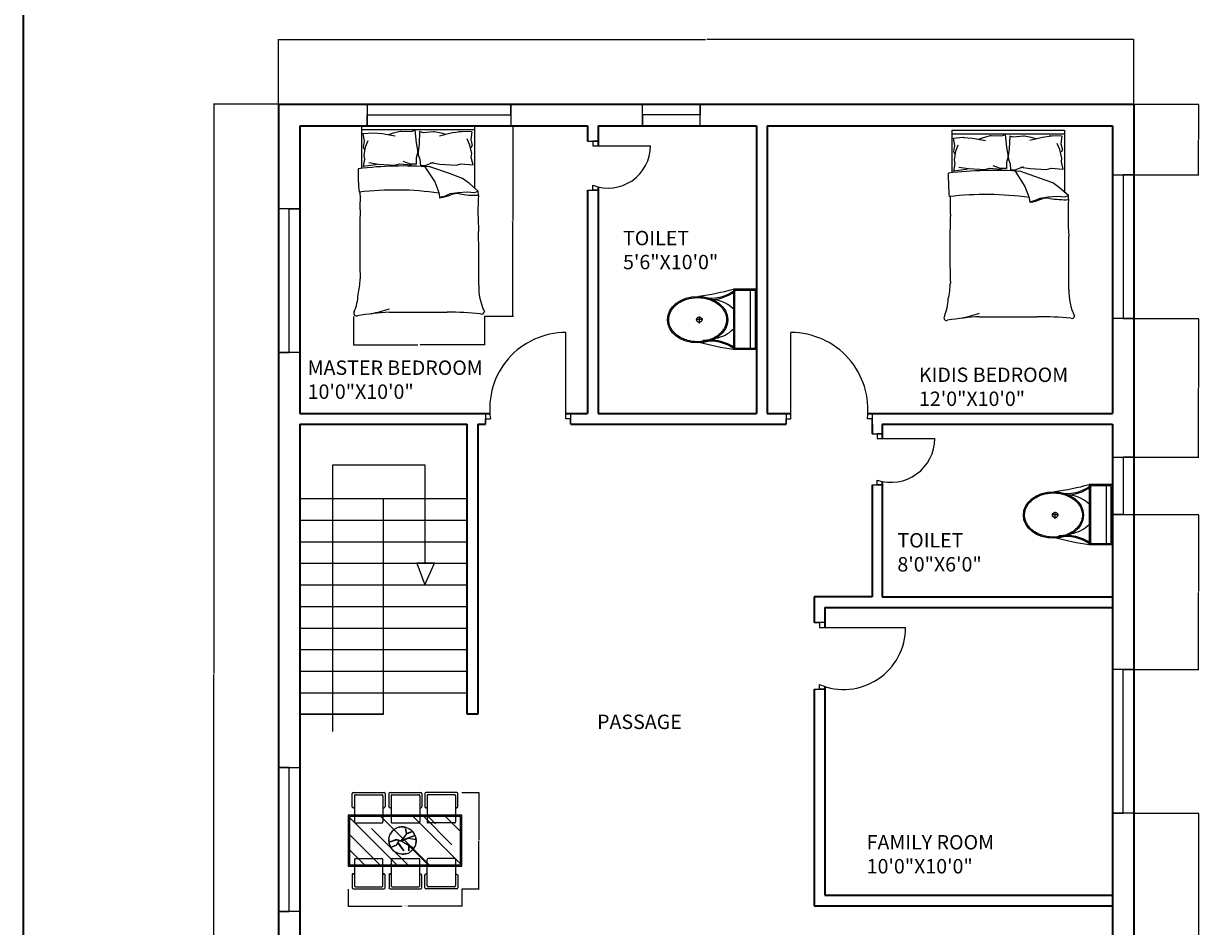
# Model space of a CAD drawing. Units: inches. Extents: x 1912 to 3731, y 1384 to 2459.
# Tile 2 of 8: x 1912 to 2405, y 1630 to 2007. Entities that reach past the tile are written whole.
import ezdxf

# ---------------------------------------------------------------- set-up
doc = ezdxf.new("R2010")
doc.units = ezdxf.units.IN
for name, color, linetype, lineweight in [('A-ANNO-DIMS', 2, 'Continuous', 18), ('A-ANNO-TTLB', 7, 'Continuous', 35), ('A-AREA-IDEN', 7, 'Continuous', 18), ('A-DOOR', 3, 'Continuous', 20), ('A-FLOR-FIXT', 9, 'Continuous', 18), ('A-FLOR-STRS', 7, 'Continuous', 18), ('A-FURN', 8, 'Continuous', 15), ('A-GLAZ', 4, 'Continuous', 18), ('A-WALL', 7, 'Continuous', 35)]:
    doc.layers.add(name, color=color, linetype=linetype, lineweight=lineweight)
doc.styles.get("Standard").update_dxf_attribs({"font": 'arial.ttf'})
doc.dimstyles.get("Standard").update_dxf_attribs({"dimtxt": 0.18, "dimasz": 0.18, "dimexe": 0.18, "dimexo": 0.0625, "dimgap": 0.09, "dimtad": 0, "dimtih": 1, "dimtoh": 1, "dimdec": 4, "dimzin": 0, "dimdsep": 46, "dimtxsty": 'Standard', "dimcen": 0.09, "dimadec": 0, "dimazin": 0, "dimtfac": 1, "dimtdec": 4, "dimtofl": 0, "dimtmove": 0, "dimatfit": 3, "dimfxl": 1, "dimtolj": 1, "dimtzin": 0, "dimarcsym": 0})

# ---------------------------------------------------------------- blocks, each defined once
blk = doc.blocks.new('A$C31115884')
for p, q in [((258, 466), (258, 523)), ((283, 498), (223, 498)), ((0, 200), (0, 0)), ((520, 200), (0, 200)), ((10, 190), (10, 10)), ((510, 190), (10, 190)), ((510, 10), (510, 190)), ((520, 0), (520, 200)), ((510, 54), (0, 54)), ((10, 10), (510, 10)), ((0, 0), (520, 0))]:
    blk.add_line(p, q)
blk.add_circle((256, 496), 23.6)
for centre, radius, start, end in [((2778, -205), 2807, 165.4549, 171.7133), ((-295, 403), 365, 324.2091, 9.3499), ((-295, 403), 375, 324.2091, 9.3499), ((139, 406), 293, 315.8436, 2.6563), ((806, 403), 365, 170.6501, 215.7909), ((3237, 905), 2807, 188.2867, 194.5451), ((384, 406), 293, 190.2774, 224.1564), ((806, 403), 375, 179.2036, 215.7909)]:
    blk.add_arc(centre, radius, start, end)
blk.add_ellipse((256, 510), major_axis=(0, -261), ratio=0.772727)
blk.add_open_spline([(256, 259), (263, 259), (270, 260), (288, 262), (299, 265), (320, 273), (330, 278), (350, 291), (360, 299), (378, 316), (386, 326), (402, 347), (409, 358), (421, 383), (427, 395), (436, 422), (440, 436), (445, 465), (447, 480), (448, 509), (448, 524), (445, 553), (443, 568), (436, 596), (432, 610), (422, 636), (416, 649), (402, 672), (395, 683), (379, 703), (370, 712), (351, 728), (341, 735), (321, 746), (310, 751), (289, 757), (278, 759), (256, 761), (245, 761), (223, 757), (212, 754), (191, 746), (181, 741), (161, 728), (151, 720), (133, 703), (125, 693), (110, 672), (103, 660), (90, 636), (85, 623), (76, 596), (72, 582), (67, 553), (66, 538), (64, 509), (65, 494), (68, 465), (70, 450), (77, 422), (81, 408), (91, 382), (97, 370), (111, 346), (118, 335), (135, 316), (144, 307), (162, 291), (172, 284), (193, 273), (203, 269), (225, 262), (236, 260), (250, 259), (253, 259), (256, 259)], degree=3, knots=[0, 0, 0, 0, 0.110105, 0.110105, 0.285049, 0.285049, 0.459994, 0.459994, 0.634938, 0.634938, 0.809882, 0.809882, 0.984827, 0.984827, 1.159771, 1.159771, 1.334715, 1.334715, 1.50966, 1.50966, 1.684604, 1.684604, 1.859549, 1.859549, 2.034493, 2.034493, 2.209437, 2.209437, 2.384382, 2.384382, 2.559326, 2.559326, 2.73427, 2.73427, 2.909215, 2.909215, 3.084159, 3.084159, 3.259103, 3.259103, 3.434048, 3.434048, 3.608992, 3.608992, 3.783936, 3.783936, 3.958881, 3.958881, 4.133825, 4.133825, 4.30877, 4.30877, 4.483714, 4.483714, 4.658658, 4.658658, 4.833603, 4.833603, 5.008547, 5.008547, 5.183491, 5.183491, 5.358436, 5.358436, 5.53338, 5.53338, 5.708324, 5.708324, 5.883269, 5.883269, 6.058213, 6.058213, 6.233158, 6.233158, 6.283185, 6.283185, 6.283185, 6.283185])
blk = doc.blocks.new('BED-DOUBLE')
for p, q in [((3.41, 61.57), (3.41, 79.35)), ((3.41, 79.35), (50.34, 79.35)), ((50.34, 79.35), (50.34, 53.22)), ((3.41, 77.85), (50.34, 77.85)), ((3.82, 76.1), (4.39, 72.97)), ((3.83, 76.07), (8.03, 76.4)), ((8.03, 76.4), (8.14, 76.38)), ((8.14, 76.38), (11.89, 76.1)), ((11.89, 76.1), (17.29, 75.1)), ((14.59, 75.67), (16.58, 76.38)), ((16.58, 76.38), (19.41, 77.09)), ((19.41, 77.09), (19.73, 77.09)), ((19.73, 77.09), (24.1, 76.95)), ((24.1, 76.95), (25.52, 77.52)), ((25.52, 77.52), (26.08, 72.26)), ((27.47, 76.9), (27.24, 71.63)), ((28.93, 76.43), (27.47, 76.9)), ((33.27, 76.84), (28.93, 76.43)), ((33.59, 76.86), (33.27, 76.84)), ((36.47, 76.33), (33.59, 76.86)), ((41.16, 76.34), (35.84, 75.01)), ((38.5, 75.74), (36.47, 76.33)), ((44.89, 76.86), (41.16, 76.34)), ((49.21, 76.84), (43.91, 76.94)), ((43.91, 76.94), (44.89, 76.86)), ((49.21, 76.84), (48.84, 73.69)), ((4.39, 72.97), (3.97, 70.42)), ((3.97, 70.42), (4.53, 69.42)), ((4.39, 67.01), (4.96, 70.56)), ((4.96, 70.56), (5.95, 73.26)), ((26.08, 72.26), (26.65, 69.14)), ((26.65, 69.14), (26.65, 67.86)), ((27.24, 71.63), (26.86, 68.47)), ((48.42, 71.24), (47.26, 73.87)), ((49.21, 67.74), (48.42, 71.24)), ((48.84, 73.69), (49.42, 71.16)), ((49.42, 71.16), (48.92, 70.14)), ((4.11, 62.32), (4.68, 65.45)), ((4.68, 65.45), (4.39, 67.01)), ((23.67, 63.38), (20.58, 64.45)), ((26.65, 67.86), (26.08, 66.01)), ((26.08, 66.01), (26.08, 63.38)), ((26.86, 68.47), (26.94, 67.2)), ((26.94, 67.2), (27.62, 65.39)), ((27.62, 65.39), (27.79, 62.76)), ((30.2, 62.91), (33.21, 64.17)), ((49.03, 66.16), (49.21, 67.74)), ((49.79, 63.08), (49.03, 66.16)), ((9.11, 63.03), (4.11, 62.32)), ((6.27, 64), (10.23, 63.35)), ((10.23, 63.35), (9.11, 63.03)), ((10.23, 63.35), (17.11, 62.93)), ((17.11, 62.93), (19.04, 63.47)), ((19.04, 63.47), (24.08, 63.08)), ((26.08, 63.38), (23.67, 63.38)), ((27.79, 62.76), (30.2, 62.91)), ((29.72, 62.28), (33.83, 55.9)), ((39.91, 59.4), (31.73, 62.28)), ((31.98, 64), (35.94, 63.35)), ((35.94, 63.35), (42.82, 62.93)), ((45.39, 57.42), (39.91, 59.4)), ((42.82, 62.93), (44.75, 63.47)), ((44.75, 63.47), (49.79, 63.08)), ((33.83, 55.9), (35.5, 51.5)), ((48.28, 55.3), (45.39, 57.42)), ((51.92, 52.1), (48.28, 55.3)), ((35.5, 51.5), (35.81, 49.52)), ((35.81, 49.52), (38.24, 50.13)), ((38.24, 50.13), (40.22, 51.04)), ((40.22, 51.04), (43.56, 51.5)), ((43.56, 51.5), (47.37, 51.8)), ((47.37, 51.8), (50.41, 51.5)), ((50.41, 51.5), (51.92, 52.1)), ((52, 50.39), (51.92, 52.1, 3.8)), ((14.79, 1.53), (38.96, 1.53))]:
    blk.add_line(p, q)
for centre, radius, start, end in [((83.63, 59.62), 81.81, 178.7218, 185.604), ((20.98, -99.43), 162, 86.0865, 96.7821), ((17.44, -74.15), 126.7, 81.7845, 96.9006), ((-164.3, 48.74), 167.05, 358.4762, 1.0082), ((35.98, 49.46), 0.181, 160.2464, 271.1377), ((30.59, 77.9), 29.12, 280.6617, 289.8806), ((42.96, 44.92), 6.11, 78.6608, 113.7384), ((50.4, 85.89), 35.53, 259.8763, 272.5657), ((178.99, 43.69), 127.17, 176.9791, 183.8365), ((476.11, 29.65), 473.64, 178.2277, 181.7185), ((-4427.7, 12.75), 4479.86, 0.00217, 0.28689), ((-26.42, 16), 29.1, 346.0648, 358.9113), ((74.79, 11.92), 22.65, 177.4714, 206.4681), ((-21.27, 10.34), 23.14, 337.9751, 356.652), ((1.07, 1.07), 1.07, 146.1736, 293.4781), ((21.04, -117.88), 119.57, 92.9958, 99.4091), ((-16.91, 102.64), 104.55, 283.3832, 287.7053), ((40.41, -129.11), 130.65, 84.4998, 90.6351), ((53.43, 1.9), 1.08, 242.6588, 356.02)]:
    blk.add_arc(centre, radius, start, end)
blk = doc.blocks.new('DINING-SET-6')
h = blk.add_hatch()
h.set_pattern_fill('AR-RROOF', color=256, scale=14.228383, angle=-45, style=0)
h.set_pattern_definition([(315, (468.26, 1216.031), (32.19516, -12.07318), [213.4257, -28.4568, 71.1419, -14.2284]), (315, (486.671, 1207.68), (3.32013, 23.4421), [42.68515, -4.6954, 85.3703, -10.6713]), (315, (481.842, 1219.553), (59.05799, -45.57627), [113.82706, -19.91974, 56.9135, -14.2284])])
h.paths.add_polyline_path([(0.59, 10.06), (46.84, 10.06), (46.84, 30.22), (0.59, 30.22)])
for p, q in [((1.68, 34.33), (1.68, 39.85)), ((2.11, 40.28), (15.01, 40.28)), ((15.44, 39.85), (15.44, 34.33)), ((17.07, 34.33), (17.07, 39.85)), ((17.49, 40.28), (30.39, 40.28)), ((30.82, 39.85), (30.82, 34.33)), ((31.99, 39.85), (31.99, 34.33)), ((45.32, 40.28), (32.42, 40.28)), ((45.75, 34.33), (45.75, 39.85)), ((2.63, 38.9), (2.63, 27.95)), ((3.06, 39.33), (14.06, 39.33)), ((14.49, 38.9), (14.49, 27.95)), ((18.01, 38.9), (18.01, 27.95)), ((18.44, 39.33), (29.45, 39.33)), ((29.87, 38.9), (29.87, 27.95)), ((32.94, 38.9), (32.94, 27.95)), ((44.37, 39.33), (33.37, 39.33)), ((44.8, 38.9), (44.8, 27.95)), ((47.43, 30.81), (0, 30.81)), ((0, 30.81), (0, 9.47)), ((46.84, 30.22), (0.59, 30.22)), ((0.59, 30.22), (0.59, 10.06)), ((2.11, 33.9), (2.2, 33.9)), ((14.91, 33.9), (15.01, 33.9)), ((17.49, 33.9), (17.59, 33.9)), ((30.3, 33.9), (30.39, 33.9)), ((32.51, 33.9), (32.42, 33.9)), ((45.32, 33.9), (45.22, 33.9)), ((46.84, 10.06), (46.84, 30.22)), ((47.43, 9.47), (47.43, 30.81)), ((3.06, 27.52), (14.06, 27.52)), ((18.44, 27.52), (29.45, 27.52)), ((19.26, 24.45), (18.96, 24.82)), ((19.6, 24.7), (19.33, 25.09)), ((19.97, 24.93), (19.73, 25.34)), ((20.34, 25.13), (20.14, 25.56)), ((20.74, 25.3), (20.57, 25.74)), ((21.14, 25.44), (21.01, 25.89)), ((21.56, 25.54), (21.46, 26)), ((21.98, 25.61), (21.92, 26.08)), ((22.41, 25.65), (22.38, 26.13)), ((22.84, 25.66), (22.85, 26.13)), ((23.26, 25.63), (23.31, 26.1)), ((23.69, 25.57), (23.77, 26.03)), ((23.93, 25.25), (24.31, 23.05)), ((24.4, 23.13), (23.93, 25.25)), ((24.11, 25.47), (24.23, 25.93)), ((24.51, 25.34), (24.67, 25.79)), ((24.91, 25.18), (25.1, 25.62)), ((25.3, 25), (25.52, 25.41)), ((25.66, 24.78), (25.92, 25.17)), ((26.01, 24.53), (26.3, 24.9)), ((44.37, 27.52), (33.37, 27.52)), ((17.24, 20.35), (16.76, 20.37)), ((17.24, 19.93), (16.77, 19.9)), ((17.26, 20.78), (16.79, 20.83)), ((17.33, 21.2), (16.86, 21.29)), ((17.42, 21.62), (16.96, 21.75)), ((20.08, 20.59), (17.07, 19.53)), ((17.07, 19.53), (20.08, 20.46)), ((17.55, 22.03), (17.1, 22.19)), ((17.71, 22.43), (17.27, 22.62)), ((17.9, 22.81), (17.48, 23.04)), ((18.12, 23.18), (17.72, 23.44)), ((18.36, 23.53), (17.99, 23.82)), ((18.64, 23.86), (18.29, 24.18)), ((18.94, 24.17), (18.61, 24.51)), ((21.3, 20.29), (20.03, 18.3)), ((22.07, 20.12), (20.08, 20.59)), ((20.08, 20.46), (22.32, 19.91)), ((20.16, 18.21), (21.35, 20.16)), ((24.31, 23.05), (22.07, 20.08)), ((27.87, 22.37), (22.07, 20.08)), ((25.33, 18.16), (22.11, 19.91)), ((22.32, 19.95), (24.82, 21.04)), ((22.36, 20.12), (24.44, 23.05)), ((22.36, 19.95), (27.32, 17.07)), ((26.51, 23.81), (24.4, 23.13)), ((24.44, 23.05), (26.51, 23.81)), ((28.08, 20.67), (24.82, 21.04)), ((25.04, 21.14), (27.87, 22.37)), ((25.04, 21.14), (28.08, 20.67)), ((26.34, 24.25), (26.66, 24.61)), ((26.65, 23.95), (26.99, 24.28)), ((26.93, 23.63), (27.3, 23.93)), ((27.19, 23.29), (27.58, 23.56)), ((27.41, 22.93), (27.83, 23.16)), ((27.61, 22.55), (28.04, 22.75)), ((27.78, 22.15), (28.22, 22.32)), ((27.92, 21.75), (28.37, 21.88)), ((28.02, 21.33), (28.49, 21.43)), ((28.1, 20.91), (28.57, 20.97)), ((28.13, 20.48), (28.61, 20.51)), ((28.14, 20.06), (28.61, 20.04)), ((17.28, 19.5), (16.81, 19.44)), ((17.35, 19.08), (16.89, 18.98)), ((17.46, 18.66), (17, 18.53)), ((17.59, 18.26), (17.15, 18.09)), ((17.76, 17.86), (17.33, 17.66)), ((17.96, 17.48), (17.55, 17.25)), ((18.19, 17.12), (17.8, 16.85)), ((20.03, 18.3), (18, 17.37)), ((18, 17.37), (20.16, 18.21)), ((18.45, 16.78), (18.08, 16.48)), ((18.73, 16.45), (18.38, 16.13)), ((19.03, 16.16), (18.72, 15.8)), ((19.36, 15.88), (19.07, 15.51)), ((19.71, 15.63), (19.45, 15.24)), ((20.08, 15.41), (19.85, 15)), ((20.46, 15.22), (20.27, 14.79)), ((20.86, 15.07), (20.7, 14.62)), ((23.21, 15.88), (20.71, 19.23)), ((20.84, 19.23), (23.21, 15.88)), ((21.27, 14.94), (21.15, 14.48)), ((21.69, 14.84), (21.6, 14.38)), ((23.39, 14.8), (23.46, 14.33)), ((23.82, 14.87), (23.91, 14.4)), ((24.23, 14.97), (24.37, 14.52)), ((24.64, 15.11), (24.81, 14.67)), ((25.03, 15.28), (25.23, 14.85)), ((25.33, 15.84), (25.33, 18.16)), ((25.43, 18.1), (25.33, 15.84)), ((25.41, 15.48), (25.65, 15.07)), ((27.32, 17.07), (25.43, 18.1)), ((25.77, 15.71), (26.04, 15.32)), ((26.12, 15.96), (26.41, 15.59)), ((26.44, 16.24), (26.76, 15.9)), ((26.74, 16.55), (27.09, 16.23)), ((27.01, 16.88), (27.39, 16.59)), ((27.26, 17.23), (27.66, 16.97)), ((27.48, 17.6), (27.89, 17.37)), ((27.67, 17.98), (28.1, 17.79)), ((27.83, 18.38), (28.27, 18.22)), ((27.95, 18.79), (28.41, 18.66)), ((28.05, 19.2), (28.52, 19.12)), ((28.11, 19.63), (28.58, 19.58)), ((0.59, 10.06), (46.84, 10.06)), ((2.63, 12.33), (2.63, 1.38)), ((3.06, 12.76), (14.06, 12.76)), ((14.49, 1.38), (14.49, 12.33)), ((18.01, 12.33), (18.01, 1.38)), ((18.44, 12.76), (29.45, 12.76)), ((22.11, 14.78), (22.06, 14.31)), ((22.54, 14.75), (22.53, 14.28)), ((22.97, 14.76), (22.99, 14.28)), ((29.87, 1.38), (29.87, 12.33)), ((32.94, 1.38), (32.94, 12.33)), ((44.37, 12.76), (33.37, 12.76)), ((44.8, 12.33), (44.8, 1.38)), ((0, 9.47), (47.43, 9.47)), ((1.68, 5.95), (1.68, 0.43)), ((2.11, 6.38), (2.21, 6.38)), ((14.92, 6.29), (15.01, 6.29)), ((15.44, 0.43), (15.44, 5.95)), ((17.07, 5.95), (17.07, 0.43)), ((17.5, 6.27), (17.59, 6.27)), ((30.3, 6.19), (30.4, 6.19)), ((30.82, 0.43), (30.82, 5.95)), ((31.99, 0.43), (31.99, 5.95)), ((32.52, 6.17), (32.42, 6.18)), ((45.32, 6.09), (45.23, 6.09)), ((45.75, 5.95), (45.75, 0.43)), ((3.06, 0.95), (14.06, 0.95)), ((18.44, 0.95), (29.45, 0.95)), ((44.37, 0.95), (33.37, 0.95)), ((2.11, 0), (15.01, 0)), ((17.49, 0), (30.39, 0)), ((45.32, 0), (32.42, 0))]:
    blk.add_line(p, q)
for centre, start, end in [((2.11, 39.85), 90, 180), ((15.01, 39.85), 0, 90), ((17.49, 39.85), 90, 180), ((30.39, 39.85), 0, 90), ((32.42, 39.85), 90, 180), ((45.32, 39.85), 0, 90), ((3.06, 38.9), 90, 180), ((14.06, 38.9), 0, 90), ((18.44, 38.9), 90, 180), ((29.45, 38.9), 0, 90), ((33.37, 38.9), 90, 180), ((44.37, 38.9), 0, 90), ((2.11, 34.33), 180, 0.104), ((14.91, 34.33), 180, 0.104), ((17.49, 34.33), 180, 270), ((17.59, 34.33), 270, 0), ((30.3, 34.33), 180, 270), ((30.39, 34.33), 270, 0), ((32.42, 34.33), 180, 270), ((32.51, 34.33), 270, 0), ((45.22, 34.33), 180, 270), ((45.32, 34.33), 270, 0), ((3.06, 27.95), 180, 270), ((14.06, 27.95), 270, 0), ((18.44, 27.95), 180, 270), ((29.45, 27.95), 270, 0), ((33.37, 27.95), 180, 270), ((44.37, 27.95), 270, 0), ((3.06, 12.33), 90, 180), ((14.06, 12.33), 0, 90), ((18.44, 12.33), 90, 180), ((29.45, 12.33), 0, 90), ((33.37, 12.33), 90, 180), ((44.37, 12.33), 0, 90), ((2.11, 5.95), 89.6202, 179.6202), ((2.2, 5.95), 359.6202, 89.6202), ((14.91, 5.86), 89.6202, 179.6202), ((15.01, 5.86), 359.6202, 89.6202), ((17.49, 5.85), 89.6202, 179.6202), ((17.59, 5.85), 359.6202, 89.6202), ((30.3, 5.76), 89.6202, 179.6202), ((30.39, 5.76), 359.6202, 89.6202), ((32.42, 5.75), 89.6202, 179.6202), ((32.51, 5.75), 359.6202, 89.6202), ((45.22, 5.66), 89.6202, 179.6202), ((45.32, 5.66), 359.6202, 89.6202), ((2.11, 0.43), 180, 270), ((3.06, 1.38), 180, 270), ((14.06, 1.38), 270, 0), ((15.01, 0.43), 270, 0), ((17.49, 0.43), 180, 270), ((18.44, 1.38), 180, 270), ((29.45, 1.38), 270, 0), ((30.39, 0.43), 270, 0), ((32.42, 0.43), 180, 270), ((33.37, 1.38), 180, 270), ((44.37, 1.38), 270, 0), ((45.32, 0.43), 270, 0)]:
    blk.add_arc(centre, 0.427, start, end)
blk = doc.blocks.new('STAIR-RETURN-GROUND')
for p, q in [((13.73, 0), (13.73, 111.26)), ((13.73, 111.26), (52.04, 111.26)), ((52.04, 111.26), (52.04, 70.24)), ((0, 97.24), (34.87, 97.24)), ((34.87, 97.24), (69.75, 97.24)), ((34.87, 7.24), (34.87, 97.12)), ((0, 88.24), (34.87, 88.24)), ((34.87, 88.24), (69.75, 88.24)), ((0, 79.24), (34.87, 79.24)), ((34.87, 79.24), (69.75, 79.24)), ((0, 70.24), (34.87, 70.24)), ((34.87, 70.24), (69.75, 70.24)), ((56.12, 70.24), (48.82, 70.24)), ((48.82, 70.24), (52.04, 61.24)), ((52.04, 61.24), (56.12, 70.24)), ((0, 61.24), (34.87, 61.24)), ((34.87, 61.24), (69.75, 61.24)), ((0, 52.24), (34.87, 52.24)), ((34.87, 52.24), (69.75, 52.24)), ((0, 43.24), (34.87, 43.24)), ((34.87, 43.24), (69.75, 43.24)), ((0, 34.24), (34.87, 34.24)), ((34.87, 34.24), (69.75, 34.24)), ((0, 25.24), (34.87, 25.24)), ((34.87, 25.24), (69.75, 25.24)), ((0, 16.24), (34.87, 16.24)), ((34.87, 7.24), (34.87, 16.24)), ((34.87, 16.24), (69.75, 16.24)), ((34.87, 7.24), (0, 7.24)), ((0, 7.24), (34.87, 7.24))]:
    blk.add_line(p, q)
blk = doc.blocks.new('DOOR-36-GF-KIDS')
for p, q in [((2, 2.25), (2, 38.25)), ((0, 4.5), (0, 0)), ((0, 0), (0, 2.25)), ((0, 2.25), (2, 2.25)), ((35.93, 2.25), (33.93, 2.25)), ((35.93, 4.5), (35.93, 0)), ((35.93, 0), (35.93, 2.25))]:
    blk.add_line(p, q)
blk.add_arc((2, 6.09), 32.16, 353.1455, 90)
blk = doc.blocks.new('DOOR-36-GF-MASTER')
for p, q in [((33.51, 2.25), (33.51, 38.25)), ((0, 4.5), (0, 0)), ((0, 0), (0, 2.25)), ((0, 2.25), (2, 2.25)), ((35.51, 2.25), (33.51, 2.25)), ((35.51, 4.5), (35.51, 0)), ((35.51, 0), (35.51, 2.25))]:
    blk.add_line(p, q)
blk.add_arc((33.51, 6.46), 31.79, 90, 187.6029)
blk = doc.blocks.new('DOOR-24-GF-ENSUITE')
for p, q in [((0, 20.44), (4.5, 20.44)), ((4.5, 20.44), (2.25, 20.44)), ((2.25, 20.44), (2.25, 18.44)), ((2.25, 18.44), (26.25, 18.44)), ((2.25, 0), (2.25, 2)), ((0, 0), (4.5, 0)), ((4.5, 0), (2.25, 0))]:
    blk.add_line(p, q)
blk.add_arc((8.62, 18.44), 17.63, 248.8218, 0)
blk = doc.blocks.new('DOOR-24-GF-BATH')
for p, q in [((0, 21.32), (4.21, 21.32)), ((4.21, 21.32), (2.1, 21.32)), ((2.1, 21.32), (2.1, 19.32)), ((2.1, 19.32), (26.1, 19.32)), ((2.1, 0), (2.1, 2)), ((0, 0), (4.21, 0)), ((4.21, 0), (2.1, 0))]:
    blk.add_line(p, q)
blk.add_arc((7.86, 19.32), 18.25, 251.6307, 0)
blk = doc.blocks.new('DOOR-36-GF-FAMILY')
for p, q in [((4.5, 27.89), (0, 27.89)), ((0, 27.89), (2.25, 27.89)), ((2.25, 27.89), (2.25, 25.89)), ((2.25, 25.89), (38.25, 25.89)), ((0, 0.04), (4.5, 0.04)), ((2.25, 0.04), (2.25, 2.04)), ((4.5, 0.04), (2.25, 0.04))]:
    blk.add_line(p, q)
blk.add_arc((12.35, 25.89), 25.9, 247.0495, 0)
blk = doc.blocks.new('WIN-PLAN-60-A')
for p, q in [((0, 9), (0, 0)), ((60, 4.5), (60, 9)), ((60, 9), (60, 0)), ((0, 0), (0, 4.5)), ((0, 4.5), (60, 4.5))]:
    blk.add_line(p, q)
blk = doc.blocks.new('WIN-PLAN-60-B')
for p, q in [((0, 60), (9, 60)), ((9, 60), (4.5, 60)), ((4.5, 60), (4.5, 0)), ((9, 0), (0, 0)), ((4.5, 0), (9, 0))]:
    blk.add_line(p, q)
blk = doc.blocks.new('WIN-PLAN-24-A')
for p, q in [((0, 24), (9, 24)), ((9, 24), (4.5, 24)), ((4.5, 24), (4.5, 0)), ((4.5, 0), (0, 0)), ((0, 0), (9, 0))]:
    blk.add_line(p, q)
blk = doc.blocks.new('*D47')
at = {"layer": 'A-ANNO-DIMS', "color": 0, "lineweight": -2, "transparency": 16777216}
for p, q in [((2104.55, 1964.13), (2116.58, 1964.13)), ((2116.4, 1963.95), (2116.4, 1924.58)), ((2116.4, 1884.85), (2116.4, 1924.22)), ((2104.55, 1884.67), (2116.58, 1884.67))]:
    blk.add_line(p, q, dxfattribs=at)
at = {"layer": 'A-ANNO-DIMS', "color": 0, "transparency": 16777216}
for points in [[(2116.37, 1963.95), (2116.43, 1963.95), (2116.4, 1964.13)], [(2116.37, 1884.85), (2116.43, 1884.85), (2116.4, 1884.67)]]:
    blk.add_solid(points, dxfattribs=at)
at = {"layer": 'Defpoints', "color": 0, "transparency": 16777216}
for p in [(2104.48, 1964.13), (2116.4, 1964.13), (2104.48, 1884.67)]:
    blk.add_point(p, dxfattribs=at)
at = {"layer": 'A-ANNO-DIMS', "color": 0, "transparency": 16777216, "insert": (2116.4, 1924.4), "char_height": 0.18, "attachment_point": 5}
blk.add_mtext('\\A1;BED 79 TYP.', dxfattribs=at)
blk = doc.blocks.new('*D48')
at = {"layer": 'A-ANNO-DIMS', "color": 0, "lineweight": -2, "transparency": 16777216}
for p, q in [((2049.89, 1884.61), (2049.89, 1872.57)), ((2104.48, 1884.61), (2104.48, 1872.57)), ((2050.07, 1872.75), (2076.66, 1872.75)), ((2104.3, 1872.75), (2077.71, 1872.75))]:
    blk.add_line(p, q, dxfattribs=at)
at = {"layer": 'A-ANNO-DIMS', "color": 0, "transparency": 16777216}
for points in [[(2050.07, 1872.78), (2050.07, 1872.72), (2049.89, 1872.75)], [(2104.3, 1872.78), (2104.3, 1872.72), (2104.48, 1872.75)]]:
    blk.add_solid(points, dxfattribs=at)
at = {"layer": 'Defpoints', "color": 0, "transparency": 16777216}
for p in [(2049.89, 1884.67), (2104.48, 1884.67), (2104.48, 1872.75)]:
    blk.add_point(p, dxfattribs=at)
at = {"layer": 'A-ANNO-DIMS', "color": 0, "transparency": 16777216, "insert": (2077.18, 1872.75), "char_height": 0.18, "attachment_point": 5}
blk.add_mtext('\\A1;55 TYP.', dxfattribs=at)
blk = doc.blocks.new('*D49')
at = {"layer": 'A-ANNO-DIMS', "color": 0, "lineweight": -2, "transparency": 16777216}
for p, q in [((2047.61, 1645.66), (2047.61, 1638.43)), ((2095.04, 1645.66), (2095.04, 1638.43)), ((2047.79, 1638.61), (2070.05, 1638.61)), ((2094.86, 1638.61), (2072.61, 1638.61))]:
    blk.add_line(p, q, dxfattribs=at)
at = {"layer": 'A-ANNO-DIMS', "color": 0, "transparency": 16777216}
for points in [[(2047.79, 1638.64), (2047.79, 1638.58), (2047.61, 1638.61)], [(2094.86, 1638.64), (2094.86, 1638.58), (2095.04, 1638.61)]]:
    blk.add_solid(points, dxfattribs=at)
at = {"layer": 'Defpoints', "color": 0, "transparency": 16777216}
for p in [(2047.61, 1645.72), (2095.04, 1645.72), (2095.04, 1638.61)]:
    blk.add_point(p, dxfattribs=at)
at = {"layer": 'A-ANNO-DIMS', "color": 0, "transparency": 16777216, "insert": (2071.33, 1638.61), "char_height": 0.18, "attachment_point": 5}
blk.add_mtext('\\A1;DINING SET 47 TYP.', dxfattribs=at)
blk = doc.blocks.new('*D50')
at = {"layer": 'A-ANNO-DIMS', "color": 0, "lineweight": -2, "transparency": 16777216}
for p, q in [((2095.1, 1686), (2102.34, 1686)), ((2102.16, 1685.82), (2102.16, 1666.04)), ((2102.16, 1645.9), (2102.16, 1665.68)), ((2095.1, 1645.72), (2102.34, 1645.72))]:
    blk.add_line(p, q, dxfattribs=at)
at = {"layer": 'A-ANNO-DIMS', "color": 0, "transparency": 16777216}
for points in [[(2102.13, 1685.82), (2102.19, 1685.82), (2102.16, 1686)], [(2102.13, 1645.9), (2102.19, 1645.9), (2102.16, 1645.72)]]:
    blk.add_solid(points, dxfattribs=at)
at = {"layer": 'Defpoints', "color": 0, "transparency": 16777216}
for p in [(2095.04, 1686), (2102.16, 1686), (2095.04, 1645.72)]:
    blk.add_point(p, dxfattribs=at)
at = {"layer": 'A-ANNO-DIMS', "color": 0, "transparency": 16777216, "insert": (2102.16, 1665.86), "char_height": 0.18, "attachment_point": 5}
blk.add_mtext('\\A1;40 TYP.', dxfattribs=at)
blk = doc.blocks.new('*D91')
at = {"layer": 'A-ANNO-DIMS', "color": 0, "lineweight": -2, "transparency": 16777216}
for p, q in [((2018.53, 1973.19), (2018.53, 2000.26)), ((2018.71, 2000.08), (2196.74, 2000.08)), ((2375.35, 2000.08), (2197.32, 2000.08)), ((2375.53, 1973.19), (2375.53, 2000.26))]:
    blk.add_line(p, q, dxfattribs=at)
at = {"layer": 'A-ANNO-DIMS', "color": 0, "transparency": 16777216}
for points in [[(2018.71, 2000.11), (2018.71, 2000.05), (2018.53, 2000.08)], [(2375.35, 2000.11), (2375.35, 2000.05), (2375.53, 2000.08)]]:
    blk.add_solid(points, dxfattribs=at)
at = {"layer": 'Defpoints', "color": 0, "transparency": 16777216}
for p in [(2375.53, 2000.08), (2018.53, 1973.13), (2375.53, 1973.13)]:
    blk.add_point(p, dxfattribs=at)
at = {"layer": 'A-ANNO-DIMS', "color": 0, "transparency": 16777216, "insert": (2197.03, 2000.08), "char_height": 0.18, "attachment_point": 5}
blk.add_mtext('\\A1;357', dxfattribs=at)
blk = doc.blocks.new('*D92')
at = {"layer": 'A-ANNO-DIMS', "color": 0, "lineweight": -2, "transparency": 16777216}
for p, q in [((2018.47, 1973.13), (1991.4, 1973.13)), ((1991.58, 1972.95), (1991.58, 1735.56)), ((1991.58, 1497.81), (1991.58, 1735.19)), ((2018.47, 1497.63), (1991.4, 1497.63))]:
    blk.add_line(p, q, dxfattribs=at)
at = {"layer": 'A-ANNO-DIMS', "color": 0, "transparency": 16777216}
for points in [[(1991.55, 1972.95), (1991.61, 1972.95), (1991.58, 1973.13)], [(1991.55, 1497.81), (1991.61, 1497.81), (1991.58, 1497.63)]]:
    blk.add_solid(points, dxfattribs=at)
at = {"layer": 'Defpoints', "color": 0, "transparency": 16777216}
for p in [(1991.58, 1973.13), (2018.53, 1973.13), (2018.53, 1497.63)]:
    blk.add_point(p, dxfattribs=at)
at = {"layer": 'A-ANNO-DIMS', "color": 0, "transparency": 16777216, "insert": (1991.58, 1735.38), "char_height": 0.18, "attachment_point": 5}
blk.add_mtext('\\A1;475.5', dxfattribs=at)
blk = doc.blocks.new('*D93')
at = {"layer": 'A-ANNO-DIMS', "color": 0, "lineweight": -2, "transparency": 16777216}
for p, q in [((2375.59, 1973.13), (2402.66, 1973.13)), ((2402.48, 1972.95), (2402.48, 1958.58)), ((2402.48, 1943.86), (2402.48, 1958.22)), ((2375.59, 1943.68), (2402.66, 1943.68))]:
    blk.add_line(p, q, dxfattribs=at)
at = {"layer": 'A-ANNO-DIMS', "color": 0, "transparency": 16777216}
for points in [[(2402.45, 1972.95), (2402.51, 1972.95), (2402.48, 1973.13)], [(2402.45, 1943.86), (2402.51, 1943.86), (2402.48, 1943.68)]]:
    blk.add_solid(points, dxfattribs=at)
at = {"layer": 'Defpoints', "color": 0, "transparency": 16777216}
for p in [(2375.53, 1973.13), (2375.53, 1943.68), (2402.48, 1943.68)]:
    blk.add_point(p, dxfattribs=at)
at = {"layer": 'A-ANNO-DIMS', "color": 0, "transparency": 16777216, "insert": (2402.48, 1958.4), "char_height": 0.18, "attachment_point": 5}
blk.add_mtext('\\A1;29.45', dxfattribs=at)
blk = doc.blocks.new('*D94')
at = {"layer": 'A-ANNO-DIMS', "color": 0, "lineweight": -2, "transparency": 16777216}
for p, q in [((2375.59, 1883.68), (2402.66, 1883.68)), ((2402.48, 1883.5), (2402.48, 1854.98)), ((2402.48, 1826.09), (2402.48, 1854.61)), ((2375.59, 1825.91), (2402.66, 1825.91))]:
    blk.add_line(p, q, dxfattribs=at)
at = {"layer": 'A-ANNO-DIMS', "color": 0, "transparency": 16777216}
for points in [[(2402.45, 1883.5), (2402.51, 1883.5), (2402.48, 1883.68)], [(2402.45, 1826.09), (2402.51, 1826.09), (2402.48, 1825.91)]]:
    blk.add_solid(points, dxfattribs=at)
at = {"layer": 'Defpoints', "color": 0, "transparency": 16777216}
for p in [(2375.53, 1883.68), (2375.53, 1825.91), (2402.48, 1825.91)]:
    blk.add_point(p, dxfattribs=at)
at = {"layer": 'A-ANNO-DIMS', "color": 0, "transparency": 16777216, "insert": (2402.48, 1854.79), "char_height": 0.18, "attachment_point": 5}
blk.add_mtext('\\A1;57.76', dxfattribs=at)
blk = doc.blocks.new('*D95')
at = {"layer": 'A-ANNO-DIMS', "color": 0, "lineweight": -2, "transparency": 16777216}
for p, q in [((2375.59, 1801.91), (2402.66, 1801.91)), ((2402.48, 1801.73), (2402.48, 1769.8)), ((2402.48, 1737.5), (2402.48, 1769.44)), ((2375.59, 1737.32), (2402.66, 1737.32))]:
    blk.add_line(p, q, dxfattribs=at)
at = {"layer": 'A-ANNO-DIMS', "color": 0, "transparency": 16777216}
for points in [[(2402.45, 1801.73), (2402.51, 1801.73), (2402.48, 1801.91)], [(2402.45, 1737.5), (2402.51, 1737.5), (2402.48, 1737.32)]]:
    blk.add_solid(points, dxfattribs=at)
at = {"layer": 'Defpoints', "color": 0, "transparency": 16777216}
for p in [(2375.53, 1801.91), (2375.53, 1737.32), (2402.48, 1737.32)]:
    blk.add_point(p, dxfattribs=at)
at = {"layer": 'A-ANNO-DIMS', "color": 0, "transparency": 16777216, "insert": (2402.48, 1769.62), "char_height": 0.18, "attachment_point": 5}
blk.add_mtext('\\A1;64.59', dxfattribs=at)
blk = doc.blocks.new('*D96')
at = {"layer": 'A-ANNO-DIMS', "color": 0, "lineweight": -2, "transparency": 16777216}
for p, q in [((2375.59, 1677.32), (2402.66, 1677.32)), ((2402.48, 1677.14), (2402.48, 1587.66)), ((2402.48, 1497.81), (2402.48, 1587.29)), ((2375.59, 1497.63), (2402.66, 1497.63))]:
    blk.add_line(p, q, dxfattribs=at)
at = {"layer": 'A-ANNO-DIMS', "color": 0, "transparency": 16777216}
for points in [[(2402.45, 1677.14), (2402.51, 1677.14), (2402.48, 1677.32)], [(2402.45, 1497.81), (2402.51, 1497.81), (2402.48, 1497.63)]]:
    blk.add_solid(points, dxfattribs=at)
at = {"layer": 'Defpoints', "color": 0, "transparency": 16777216}
for p in [(2375.53, 1677.32), (2375.53, 1497.63), (2402.48, 1497.63)]:
    blk.add_point(p, dxfattribs=at)
at = {"layer": 'A-ANNO-DIMS', "color": 0, "transparency": 16777216, "insert": (2402.48, 1587.47), "char_height": 0.18, "attachment_point": 5}
blk.add_mtext('\\A1;179.7', dxfattribs=at)

msp = doc.modelspace()

# ---------------------------------------------------------------- linework, layer by layer
at = {"layer": 'A-ANNO-TTLB'}
msp.add_lwpolyline([(1912.2029, 2458.5537), (3720.218, 2458.5537), (3720.218, 1383.9599), (1912.2029, 1383.9599)], close=True, dxfattribs=at)
at = {"layer": 'A-WALL'}
for p, q in [((2018.5308, 1973.1258), (2018.5308, 1497.6258)), ((2018.5308, 1973.1258), (2018.5308, 1497.6258)), ((2018.5308, 1973.1258), (2375.5308, 1973.1258)), ((2375.5308, 1973.1258), (2375.5308, 1497.6258)), ((2027.5308, 1964.1258), (2147.5308, 1964.1258)), ((2027.5308, 1964.1258), (2027.5308, 1844.1258)), ((2147.5308, 1964.1258), (2147.5308, 1957.7644)), ((2152.0308, 1964.1258), (2152.0308, 1955.7644)), ((2152.0308, 1964.1258), (2218.0308, 1964.1258)), ((2218.0308, 1964.1258), (2218.0308, 1844.1258)), ((2222.5308, 1964.1258), (2222.5308, 1844.1258)), ((2222.5308, 1964.1258), (2366.5308, 1964.1258)), ((2366.5308, 1964.1258), (2366.5308, 1844.1258)), ((2147.5308, 1937.3245), (2147.5308, 1844.1258)), ((2152.0308, 1938.6218), (2152.0308, 1844.1258)), ((2027.5308, 1844.1258), (2106.7542, 1844.1258)), ((2138.4875, 1844.1258), (2147.5308, 1844.1258)), ((2152.0308, 1844.1258), (2218.0308, 1844.1258)), ((2222.5308, 1844.1258), (2232.3891, 1844.1258)), ((2264.5114, 1844.1258), (2366.5308, 1844.1258)), ((2027.5308, 1839.6258), (2097.2773, 1839.6258)), ((2027.5308, 1839.6258), (2027.5308, 1506.6258)), ((2097.2773, 1718.5838), (2097.2773, 1839.6258)), ((2101.7773, 1839.6258), (2101.7773, 1718.5838)), ((2101.7773, 1839.6258), (2104.9735, 1839.6258)), ((2140.4875, 1839.6258), (2230.3891, 1839.6258)), ((2266.3208, 1839.6258), (2266.3208, 1835.6488)), ((2270.5308, 1839.6258), (2366.5308, 1839.6258)), ((2270.5308, 1839.6258), (2270.5308, 1833.6488)), ((2366.5308, 1839.6258), (2366.5308, 1506.6258)), ((2266.3208, 1814.3297), (2266.3208, 1767.6258)), ((2270.5308, 1815.7678), (2270.5308, 1767.6258)), ((2242.0308, 1767.6258), (2242.0308, 1756.8604)), ((2266.3208, 1767.6258), (2242.0308, 1767.6258)), ((2242.0308, 1767.6258), (2242.0308, 1763.1258)), ((2270.5308, 1767.6258), (2366.5308, 1767.6258)), ((2246.5308, 1763.1258), (2266.3208, 1763.1258)), ((2246.5308, 1763.1258), (2246.5308, 1754.8604)), ((2266.3208, 1763.1258), (2366.5308, 1763.1258)), ((2246.5308, 1730.178), (2246.5308, 1643.1258)), ((2242.0308, 1729.0101), (2242.0308, 1638.6258)), ((2101.7773, 1718.5838), (2097.2773, 1718.5838)), ((2246.5308, 1643.1258), (2366.5308, 1643.1258)), ((2242.0308, 1638.6258), (2366.5308, 1638.6258))]:
    msp.add_line(p, q, dxfattribs=at)

# ---------------------------------------------------------------- block references
at = {"layer": 'A-DOOR'}
for name, p in [('DOOR-24-GF-ENSUITE', (2147.531, 1937.325)), ('DOOR-36-GF-MASTER', (2104.973, 1839.626)), ('DOOR-36-GF-KIDS', (2230.389, 1839.626)), ('DOOR-24-GF-BATH', (2266.321, 1814.33)), ('DOOR-36-GF-FAMILY', (2242.031, 1728.971))]:
    msp.add_blockref(name, p, dxfattribs=at)
at = {"layer": 'A-FLOR-FIXT', "xscale": 0.048164045903398, "yscale": 0.048164045903398, "zscale": 0.048164045903398, "rotation": 89.99999999999991}
for p in [(2218.0308, 1870.8856), (2366.5308, 1789.3899)]:
    msp.add_blockref('A$C31115884', p, dxfattribs=at)
at = {"layer": 'A-FLOR-STRS'}
msp.add_blockref('STAIR-RETURN-GROUND', (2027.531, 1711.346), dxfattribs=at)
at = {"layer": 'A-FURN'}
for name, p in [('BED-DOUBLE', (2049.971, 1884.774)), ('BED-DOUBLE', (2296.2458, 1882.9187)), ('DINING-SET-6', (2047.614, 1645.723))]:
    msp.add_blockref(name, p, dxfattribs=at)
at = {"layer": 'A-GLAZ'}
for name, p in [('WIN-PLAN-60-A', (2055.5628, 1964.126)), ('WIN-PLAN-60-B', (2366.531, 1883.676)), ('WIN-PLAN-24-A', (2366.531, 1801.913))]:
    msp.add_blockref(name, p, dxfattribs=at)
at = {"layer": 'A-GLAZ', "extrusion": (0, 0, -1), "zscale": -1, "rotation": 90}
for name, p in [('WIN-PLAN-24-A', (-2170.4876, 1964.126)), ('WIN-PLAN-60-A', (-2018.531, 1869.4675)), ('WIN-PLAN-60-A', (-2366.531, 1677.3214))]:
    msp.add_blockref(name, p, dxfattribs=at)
at = {"layer": 'A-GLAZ', "rotation": 180}
msp.add_blockref('WIN-PLAN-60-B', (2027.5305, 1696.3403), dxfattribs=at)

# ---------------------------------------------------------------- texts
at = {"layer": 'A-AREA-IDEN', "char_height": 6, "attachment_point": 1}
for s, width, insert in [('TOILET\\P5\'6"X10\'0"', 95.120473, (2162.3397, 1920.2715)), ('MASTER BEDROOM\\P10\'0"X10\'0"', 128.861593, (2030.7213, 1866.1989)), ('KIDIS BEDROOM\\P12\'0"X10\'0"', 115.981433, (2285.835, 1863.2336)), ('TOILET\\P8\'0"X6\'0"', 93.474207, (2276.8373, 1794.1798)), ('PASSAGE', 152.030801, (2151.5104, 1718.4488)), ('FAMILY ROOM \\P10\'0"X10\'0"', 123.70951, (2264.0177, 1668.2092))]:
    msp.add_mtext_dynamic_manual_height_columns(s, width=width, gutter_width=12.5, heights=[0], dxfattribs=dict(at, insert=insert))

# ---------------------------------------------------------------- dimensions: what is measured, and where the dimension line sits
at = {"layer": 'A-ANNO-DIMS'}
dim = msp.add_linear_dim(base=(2375.5308, 2000.0758), p1=(2018.5308, 1973.1258), p2=(2375.5308, 1973.1258), dimstyle='Standard', override={"dimdec": 0, "dimlfac": 1, "dimrnd": 0, "dimzin": 0, "dimdsep": 46, "dimlunit": 2}, dxfattribs=at)
dim.commit()
dim.dimension.update_dxf_attribs({"geometry": '*D91', "text_midpoint": (2197.0308, 2000.0758)})
for base, p1, p2, override, picture, middle in [((1991.5808, 1973.1258), (2018.5308, 1497.6258), (2018.5308, 1973.1258), {"dimdec": 1, "dimlfac": 1, "dimrnd": 0, "dimzin": 0, "dimdsep": 46, "dimlunit": 2}, '*D92', (1991.5808, 1735.3758)), ((2402.4808, 1943.6759), (2375.5308, 1973.1258), (2375.5308, 1943.6759), {"dimdec": 2, "dimlfac": 1, "dimrnd": 0, "dimzin": 0, "dimdsep": 46, "dimlunit": 2}, '*D93', (2402.4808, 1958.4008)), ((2402.4808, 1825.9126), (2375.5308, 1883.6759), (2375.5308, 1825.9126), {"dimdec": 2, "dimlfac": 1, "dimrnd": 0, "dimzin": 0, "dimdsep": 46, "dimlunit": 2}, '*D94', (2402.4808, 1854.7942)), ((2402.4808, 1737.3213), (2375.5308, 1801.9126), (2375.5308, 1737.3213), {"dimdec": 2, "dimlfac": 1, "dimrnd": 0, "dimzin": 0, "dimdsep": 46, "dimlunit": 2}, '*D95', (2402.4808, 1769.6169)), ((2402.4808, 1497.6258), (2375.5308, 1677.3213), (2375.5308, 1497.6258), {"dimdec": 1, "dimlfac": 1, "dimrnd": 0, "dimzin": 0, "dimdsep": 46, "dimlunit": 2}, '*D96', (2402.4808, 1587.4735))]:
    dim = msp.add_linear_dim(base=base, p1=p1, p2=p2, angle=90, dimstyle='Standard', override=override, dxfattribs=at)
    dim.commit()
    dim.dimension.update_dxf_attribs({"geometry": picture, "text_midpoint": middle})
for base, p1, p2, text, picture, middle in [((2116.4014, 1964.1258), (2104.4831, 1884.6707), (2104.4831, 1964.1258), 'BED <> TYP.', '*D47', (2116.4014, 1924.3982)), ((2102.1563, 1686.0033), (2095.0421, 1645.7228), (2095.0421, 1686.0033), '<> TYP.', '*D50', (2102.1563, 1665.8631))]:
    dim = msp.add_linear_dim(base=base, p1=p1, p2=p2, angle=90, text=text, dimstyle='Standard', override={"dimdec": 0, "dimlfac": 1, "dimrnd": 0, "dimzin": 0, "dimdsep": 46, "dimlunit": 2}, dxfattribs=at)
    dim.commit()
    dim.dimension.update_dxf_attribs({"geometry": picture, "text_midpoint": middle})
for base, p1, p2, text, picture, middle in [((2104.4831, 1872.7524), (2049.8865, 1884.6707), (2104.4831, 1884.6707), '<> TYP.', '*D48', (2077.1848, 1872.7524)), ((2095.0421, 1638.6087), (2047.6142, 1645.7228), (2095.0421, 1645.7228), 'DINING SET <> TYP.', '*D49', (2071.3282, 1638.6087))]:
    dim = msp.add_linear_dim(base=base, p1=p1, p2=p2, text=text, dimstyle='Standard', override={"dimdec": 0, "dimlfac": 1, "dimrnd": 0, "dimzin": 0, "dimdsep": 46, "dimlunit": 2}, dxfattribs=at)
    dim.commit()
    dim.dimension.update_dxf_attribs({"geometry": picture, "text_midpoint": middle})

doc.saveas('drawing.dxf')
